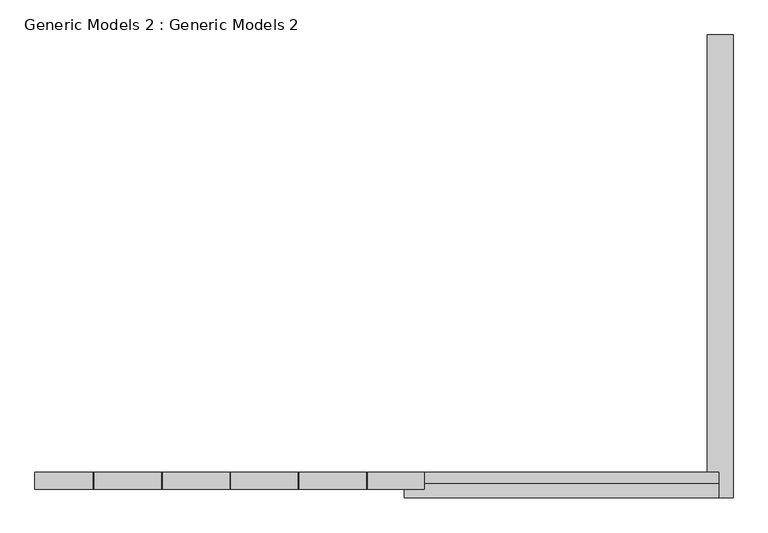
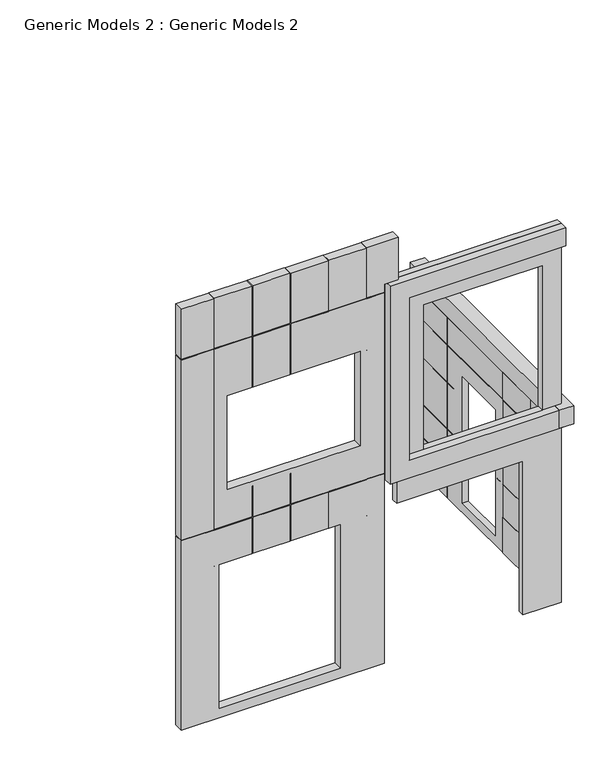
"""IFC4 building model written with IfcOpenShell, lengths in millimetres: proxy geometry, Generic Models 2 : Generic Models 2."""

from ifc_helpers import new_model, si_unit, frame, origin, place, context, project, spatial, polyline, outline, extrude, source, transform, mapped, element, save


def generic_models_2_generic_models_2_1e037190(model_context):
    return source(origin(), model_context, "Body", "SweptSolid", [
        extrude(outline(polyline([(-7046.3953834, 4640.1176199), (-7046.3953834, 511.5262137), (-7274.9953834, 511.5262137), (-7274.9953834, 4640.1176199), (-7046.3953834, 4640.1176199)])), frame((0.0, 0.0, 2895.6), z_axis=(0.0, 0.0, 1.0), x_axis=(1.0, 0.0, 0.0)), (0.0, 0.0, 1.0), 304.8),
        extrude(outline(polyline([(-7173.3953834, 4640.1176199), (-7173.3953834, 4422.4373011), (-7274.9953834, 4422.4373011), (-7274.9953834, 4640.1176199), (-7173.3953834, 4640.1176199)])), frame((0.0, 0.0, 2438.4), z_axis=(0.0, 0.0, 1.0), x_axis=(1.0, 0.0, 0.0)), (0.0, 0.0, 1.0), 457.2),
        extrude(outline(polyline([(4640.1176199, -152.4), (4422.4373011, -152.4), (4422.4373011, 444.5), (4595.6676199, 444.5), (4595.6676199, 457.2), (4422.4373011, 457.2), (4422.4373011, 1003.3), (4596.7590262, 1003.3), (4596.7590262, 1016.0), (4422.4373011, 1016.0), (4422.4373011, 1790.7), (4621.0676199, 1790.7), (4621.0676199, 1803.4), (4422.4373011, 1803.4), (4422.4373011, 2425.7), (4640.1176199, 2425.7), (4640.1176199, -152.4)])), frame((-7274.9953834, 0.0, 0.0), z_axis=(1.0, 0.0, 0.0), x_axis=(0.0, 1.0, 0.0)), (0.0, 0.0, 1.0), 101.6),
        extrude(outline(polyline([(-7173.3953834, 740.1262137), (-7274.9953834, 740.1262137), (-7274.9953834, 1310.9373011), (-7173.3953834, 1310.9373011), (-7173.3953834, 740.1262137)])), frame((0.0, 0.0, -152.4), z_axis=(0.0, 0.0, 1.0), x_axis=(1.0, 0.0, 0.0)), (0.0, 0.0, 1.0), 596.9),
        extrude(outline(polyline([(-7173.3953834, 1310.9373011), (-7173.3953834, 740.1262137), (-7274.9953834, 740.1262137), (-7274.9953834, 1310.9373011), (-7173.3953834, 1310.9373011)])), frame((0.0, 0.0, 2438.4), z_axis=(0.0, 0.0, 1.0), x_axis=(1.0, 0.0, 0.0)), (0.0, 0.0, 1.0), 457.2),
        extrude(outline(polyline([(-7173.3953834, 2072.9373011), (-7173.3953834, 1323.6373011), (-7274.9953834, 1323.6373011), (-7274.9953834, 2072.9373011), (-7173.3953834, 2072.9373011)])), frame((0.0, 0.0, 2438.4), z_axis=(0.0, 0.0, 1.0), x_axis=(1.0, 0.0, 0.0)), (0.0, 0.0, 1.0), 457.2),
        extrude(outline(polyline([(-7173.3953834, 2072.9373011), (-7173.3953834, 1323.6373011), (-7274.9953834, 1323.6373011), (-7274.9953834, 2072.9373011), (-7173.3953834, 2072.9373011)])), frame((0.0, 0.0, -152.4), z_axis=(0.0, 0.0, 1.0), x_axis=(1.0, 0.0, 0.0)), (0.0, 0.0, 1.0), 596.9),
        extrude(outline(polyline([(-7173.3953834, 3596.9373011), (-7173.3953834, 2085.6373011), (-7274.9953834, 2085.6373011), (-7274.9953834, 3596.9373011), (-7173.3953834, 3596.9373011)])), frame((0.0, 0.0, 2438.4), z_axis=(0.0, 0.0, 1.0), x_axis=(1.0, 0.0, 0.0)), (0.0, 0.0, 1.0), 457.2),
        extrude(outline(polyline([(3596.9373011, -152.4), (2085.6373011, -152.4), (2085.6373011, 444.5), (2252.5176199, 444.5), (2252.5176199, 457.2), (2085.6373011, 457.2), (2085.6373011, 1003.3), (2227.1176199, 1003.3), (2227.1176199, 1016.0), (2085.6373011, 1016.0), (2085.6373011, 1790.7), (2252.5176199, 1790.7), (2252.5176199, 1803.4), (2085.6373011, 1803.4), (2085.6373011, 2425.7), (3596.9373011, 2425.7), (3596.9373011, 1803.4), (3280.1262137, 1803.4), (3280.1262137, 1790.7), (3596.9373011, 1790.7), (3596.9373011, 1016.0), (3230.4176199, 1016.0), (3230.4176199, 1003.3), (3596.9373011, 1003.3), (3596.9373011, 457.2), (3280.1262137, 457.2), (3280.1262137, 444.5), (3596.9373011, 444.5), (3596.9373011, -152.4)]), holes=[polyline([(3205.0176199, 0.0), (3205.0176199, 2133.6), (2290.6176199, 2133.6), (2290.6176199, 0.0), (3205.0176199, 0.0)])]), frame((-7274.9953834, 0.0, 0.0), z_axis=(1.0, 0.0, 0.0), x_axis=(0.0, 1.0, 0.0)), (0.0, 0.0, 1.0), 101.6),
        extrude(outline(polyline([(-7173.3953834, 4409.7373011), (-7173.3953834, 3609.6373011), (-7274.9953834, 3609.6373011), (-7274.9953834, 4409.7373011), (-7173.3953834, 4409.7373011)])), frame((0.0, 0.0, 2438.4), z_axis=(0.0, 0.0, 1.0), x_axis=(1.0, 0.0, 0.0)), (0.0, 0.0, 1.0), 457.2),
        extrude(outline(polyline([(-7173.3953834, 4409.7373011), (-7173.3953834, 3609.6373011), (-7274.9953834, 3609.6373011), (-7274.9953834, 4409.7373011), (-7173.3953834, 4409.7373011)])), frame((0.0, 0.0, -152.4), z_axis=(0.0, 0.0, 1.0), x_axis=(1.0, 0.0, 0.0)), (0.0, 0.0, 1.0), 596.9),
        extrude(outline(polyline([(-7173.3953834, 1310.9373011), (-7173.3953834, 740.1262137), (-7274.9953834, 740.1262137), (-7274.9953834, 1310.9373011), (-7173.3953834, 1310.9373011)])), frame((0.0, 0.0, 1803.4), z_axis=(0.0, 0.0, 1.0), x_axis=(1.0, 0.0, 0.0)), (0.0, 0.0, 1.0), 622.3),
        extrude(outline(polyline([(-7173.3953834, 1310.9373011), (-7173.3953834, 740.1262137), (-7274.9953834, 740.1262137), (-7274.9953834, 1310.9373011), (-7173.3953834, 1310.9373011)])), frame((0.0, 0.0, 1016.0), z_axis=(0.0, 0.0, 1.0), x_axis=(1.0, 0.0, 0.0)), (0.0, 0.0, 1.0), 774.7),
        extrude(outline(polyline([(-7173.3953834, 1310.9373011), (-7173.3953834, 740.1262137), (-7274.9953834, 740.1262137), (-7274.9953834, 1310.9373011), (-7173.3953834, 1310.9373011)])), frame((0.0, 0.0, 457.2), z_axis=(0.0, 0.0, 1.0), x_axis=(1.0, 0.0, 0.0)), (0.0, 0.0, 1.0), 546.1),
        extrude(outline(polyline([(-7173.3953834, 2072.9373011), (-7173.3953834, 1323.6373011), (-7274.9953834, 1323.6373011), (-7274.9953834, 2072.9373011), (-7173.3953834, 2072.9373011)])), frame((0.0, 0.0, 1803.4), z_axis=(0.0, 0.0, 1.0), x_axis=(1.0, 0.0, 0.0)), (0.0, 0.0, 1.0), 622.3),
        extrude(outline(polyline([(-7173.3953834, 2072.9373011), (-7173.3953834, 1323.6373011), (-7274.9953834, 1323.6373011), (-7274.9953834, 2072.9373011), (-7173.3953834, 2072.9373011)])), frame((0.0, 0.0, 1016.0), z_axis=(0.0, 0.0, 1.0), x_axis=(1.0, 0.0, 0.0)), (0.0, 0.0, 1.0), 774.7),
        extrude(outline(polyline([(-7173.3953834, 2072.9373011), (-7173.3953834, 1323.6373011), (-7274.9953834, 1323.6373011), (-7274.9953834, 2072.9373011), (-7173.3953834, 2072.9373011)])), frame((0.0, 0.0, 457.2), z_axis=(0.0, 0.0, 1.0), x_axis=(1.0, 0.0, 0.0)), (0.0, 0.0, 1.0), 546.1),
        extrude(outline(polyline([(-7173.3953834, 4409.7373011), (-7173.3953834, 3609.6373011), (-7274.9953834, 3609.6373011), (-7274.9953834, 4409.7373011), (-7173.3953834, 4409.7373011)])), frame((0.0, 0.0, 1803.4), z_axis=(0.0, 0.0, 1.0), x_axis=(1.0, 0.0, 0.0)), (0.0, 0.0, 1.0), 622.3),
        extrude(outline(polyline([(-7173.3953834, 4409.7373011), (-7173.3953834, 3609.6373011), (-7274.9953834, 3609.6373011), (-7274.9953834, 4409.7373011), (-7173.3953834, 4409.7373011)])), frame((0.0, 0.0, 1016.0), z_axis=(0.0, 0.0, 1.0), x_axis=(1.0, 0.0, 0.0)), (0.0, 0.0, 1.0), 774.7),
        extrude(outline(polyline([(-7173.3953834, 4409.7373011), (-7173.3953834, 3609.6373011), (-7274.9953834, 3609.6373011), (-7274.9953834, 4409.7373011), (-7173.3953834, 4409.7373011)])), frame((0.0, 0.0, 457.2), z_axis=(0.0, 0.0, 1.0), x_axis=(1.0, 0.0, 0.0)), (0.0, 0.0, 1.0), 546.1),
        extrude(outline(polyline([(-152.4, -7784.2297584), (-152.4, -7173.3953834), (6248.4, -7173.3953834), (6248.4, -9803.5297584), (2438.4, -9803.5297584), (2438.4, -7784.2297584), (-152.4, -7784.2297584)]), holes=[polyline([(3200.4, -9371.7297584), (5638.8, -9371.7297584), (5638.8, -7478.1953834), (3200.4, -7478.1953834), (3200.4, -9371.7297584)])]), frame((0.0, 638.5262137, 0.0), z_axis=(0.0, 1.0, 0.0), x_axis=(0.0, 0.0, 1.0)), (0.0, 0.0, 1.0), 101.6),
        extrude(outline(polyline([(3200.4, -9676.5297584), (5943.6, -9676.5297584), (5943.6, -7173.3953834), (6248.4, -7173.3953834), (6248.4, -9981.3297584), (2895.6, -9981.3297584), (2895.6, -7173.3953834), (3200.4, -7173.3953834), (3200.4, -9676.5297584)])), frame((0.0, 511.5262137, 0.0), z_axis=(0.0, 1.0, 0.0), x_axis=(0.0, 0.0, 1.0)), (0.0, 0.0, 1.0), 127.0),
        extrude(outline(polyline([(-152.4, -13274.9953834), (-152.4, -10032.1297584), (3048.0, -10032.1297584), (3048.0, -10307.0416836), (2438.4, -10307.0416836), (2438.4, -10319.7416836), (3048.0, -10319.7416836), (3048.0, -10916.6416836), (2438.4, -10916.6416836), (2438.4, -10722.2953834), (0.0, -10722.2953834), (0.0, -12678.0953834), (2438.4, -12678.0953834), (2438.4, -12148.5416836), (3048.0, -12148.5416836), (3048.0, -12745.4416836), (2438.4, -12745.4416836), (2438.4, -12758.1416836), (3048.0, -12758.1416836), (3048.0, -13274.9953834), (-152.4, -13274.9953834)])), frame((0.0, 587.7262137, 0.0), z_axis=(0.0, 1.0, 0.0), x_axis=(0.0, 0.0, 1.0)), (0.0, 0.0, 1.0), 152.4),
        extrude(outline(polyline([(5252.1648635, -10417.4953834), (3657.6, -10417.4953834), (3657.6, -12551.0953834), (5252.1648635, -12551.0953834), (5252.1648635, -11538.9416836), (6104.0211586, -11538.9416836), (6104.0211586, -12135.8416836), (5252.7809792, -12135.8416836), (5252.7809792, -12148.5416836), (6104.0211586, -12148.5416836), (6104.0211586, -12745.4416836), (3060.7, -12745.4416836), (3060.7, -12148.5416836), (3584.0619583, -12148.5416836), (3584.0619583, -12135.8416836), (3060.7, -12135.8416836), (3060.7, -11538.9416836), (3584.0619583, -11538.9416836), (3584.0619583, -11526.2416836), (3060.7, -11526.2416836), (3060.7, -10929.3416836), (3584.0619583, -10929.3416836), (3584.0619583, -10916.6416836), (3060.7, -10916.6416836), (3060.7, -10319.7416836), (3584.0619583, -10319.7416836), (3584.0619583, -10307.0416836), (3060.7, -10307.0416836), (3060.7, -10032.1297584), (6104.0211586, -10032.1297584), (6104.0211586, -10307.0416836), (5233.7309792, -10307.0416836), (5233.7309792, -10319.7416836), (6104.0211586, -10319.7416836), (6104.0211586, -10916.6416836), (5254.3684792, -10916.6416836), (5254.3684792, -10929.3416836), (6104.0211586, -10929.3416836), (6104.0211586, -11526.2416836), (5252.1648635, -11526.2416836), (5252.1648635, -10417.4953834)])), frame((0.0, 587.7262137, 0.0), z_axis=(0.0, 1.0, 0.0), x_axis=(0.0, 0.0, 1.0)), (0.0, 0.0, 1.0), 152.4),
        extrude(outline(polyline([(6248.4, -10032.1297584), (6248.4, -9803.5297584), (6962.2619583, -9803.5297584), (6962.2619583, -10307.0416836), (6116.7211586, -10307.0416836), (6116.7211586, -10032.1297584), (6248.4, -10032.1297584)])), frame((0.0, 587.7262137, 0.0), z_axis=(0.0, 1.0, 0.0), x_axis=(0.0, 0.0, 1.0)), (0.0, 0.0, 1.0), 152.4),
        extrude(outline(polyline([(-10319.7416836, 587.7262137), (-10916.6416836, 587.7262137), (-10916.6416836, 740.1262137), (-10319.7416836, 740.1262137), (-10319.7416836, 587.7262137)])), frame((0.0, 0.0, 6116.7211586), z_axis=(0.0, 0.0, 1.0), x_axis=(1.0, 0.0, 0.0)), (0.0, 0.0, 1.0), 845.5407997),
        extrude(outline(polyline([(-10929.3416836, 587.7262137), (-11526.2416836, 587.7262137), (-11526.2416836, 740.1262137), (-10929.3416836, 740.1262137), (-10929.3416836, 587.7262137)])), frame((0.0, 0.0, 6116.7211586), z_axis=(0.0, 0.0, 1.0), x_axis=(1.0, 0.0, 0.0)), (0.0, 0.0, 1.0), 845.5407997),
        extrude(outline(polyline([(-11538.9416836, 587.7262137), (-12135.8416836, 587.7262137), (-12135.8416836, 740.1262137), (-11538.9416836, 740.1262137), (-11538.9416836, 587.7262137)])), frame((0.0, 0.0, 6116.7211586), z_axis=(0.0, 0.0, 1.0), x_axis=(1.0, 0.0, 0.0)), (0.0, 0.0, 1.0), 845.5407997),
        extrude(outline(polyline([(-12148.5416836, 587.7262137), (-12745.4416836, 587.7262137), (-12745.4416836, 740.1262137), (-12148.5416836, 740.1262137), (-12148.5416836, 587.7262137)])), frame((0.0, 0.0, 6116.7211586), z_axis=(0.0, 0.0, 1.0), x_axis=(1.0, 0.0, 0.0)), (0.0, 0.0, 1.0), 845.5407997),
        extrude(outline(polyline([(-12758.1416836, 587.7262137), (-13274.9953834, 587.7262137), (-13274.9953834, 740.1262137), (-12758.1416836, 740.1262137), (-12758.1416836, 587.7262137)])), frame((0.0, 0.0, 6116.7211586), z_axis=(0.0, 0.0, 1.0), x_axis=(1.0, 0.0, 0.0)), (0.0, 0.0, 1.0), 845.5407997),
        extrude(outline(polyline([(-11538.9416836, 587.7262137), (-12135.8416836, 587.7262137), (-12135.8416836, 740.1262137), (-11538.9416836, 740.1262137), (-11538.9416836, 587.7262137)])), frame((0.0, 0.0, 2438.4), z_axis=(0.0, 0.0, 1.0), x_axis=(1.0, 0.0, 0.0)), (0.0, 0.0, 1.0), 609.6),
        extrude(outline(polyline([(-10929.3416836, 587.7262137), (-11526.2416836, 587.7262137), (-11526.2416836, 740.1262137), (-10929.3416836, 740.1262137), (-10929.3416836, 587.7262137)])), frame((0.0, 0.0, 2438.4), z_axis=(0.0, 0.0, 1.0), x_axis=(1.0, 0.0, 0.0)), (0.0, 0.0, 1.0), 609.6),
        extrude(outline(polyline([(-12758.1416836, 587.7262137), (-13274.9953834, 587.7262137), (-13274.9953834, 740.1262137), (-12758.1416836, 740.1262137), (-12758.1416836, 587.7262137)])), frame((0.0, 0.0, 3060.7), z_axis=(0.0, 0.0, 1.0), x_axis=(1.0, 0.0, 0.0)), (0.0, 0.0, 1.0), 3043.3211586),
    ])


if __name__ == "__main__":
    model = new_model("IFC4")
    model_context = context("Model", 3, world=origin())
    ifc_project = project(units=[si_unit("LENGTHUNIT", "METRE", prefix="MILLI")], contexts=[model_context])
    site = spatial("IfcSite", under=ifc_project)
    building = spatial("IfcBuilding", under=site)
    placement = place(None, origin())
    generic_models_2_generic_models_2_shape = generic_models_2_generic_models_2_1e037190(model_context)
    element("IfcBuildingElementProxy", 1, Name="Generic Models 2 : Generic Models 2", ObjectType="Generic Models 2 : Generic Models 2", at=placement, inside=building, context=model_context, shape_type="MappedRepresentation", body=[
        mapped(generic_models_2_generic_models_2_shape, transform((0.0, 0.0, 0.0), x_axis=(1.0, 0.0, 0.0), y_axis=(0.0, 1.0, 0.0), z_axis=(0.0, 0.0, 1.0))),
    ])
    save(model, "model.ifc")

# Revit data of these elements
# Element 1 (IfcBuildingElementProxy, "Generic Models 2 : Generic Models 2")
#   Materials on its faces: "Damp-proofing", "Asphalt, Pavement, Light Grey"
# Materials
#   "Damp-proofing": class "Generic", colour RGB 127 127 127, transparency 0, Description = "Damp-proofing", Cost = 0
#   "Asphalt, Pavement, Light Grey": class "Generic", colour RGB 120 120 120, transparency 0, Description = "Asphalt or tarmac paving", Cost = 0
